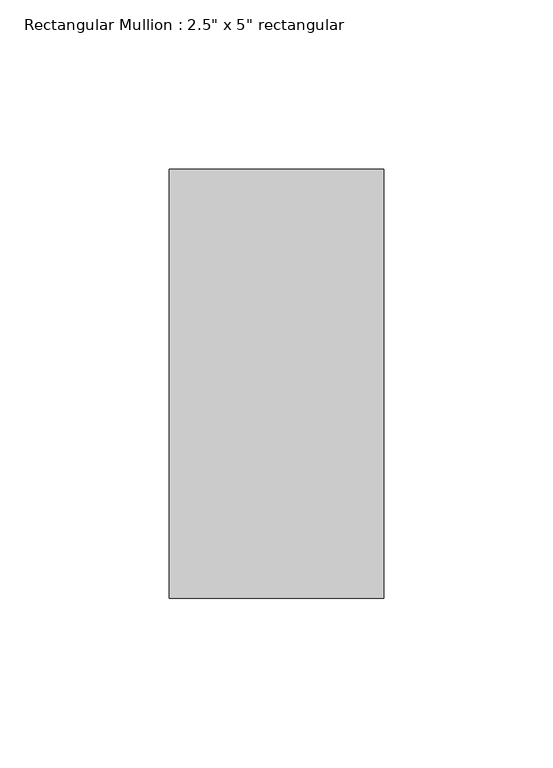
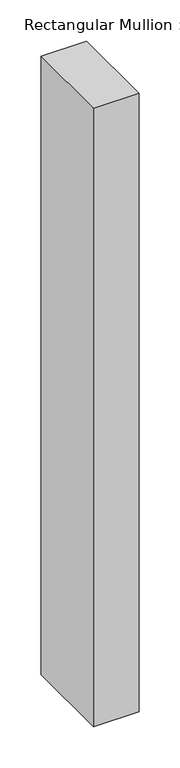
"""IFC4 building model written with IfcOpenShell, lengths in millimetres: member geometry."""

from ifc_helpers import new_model, si_unit, frame, origin, place, context, project, spatial, polyline, outline, extrude, source, transform, mapped, element, save


def member_410c6227(model_context):
    return source(origin(), model_context, "Body", "SweptSolid", [
        extrude(outline(polyline([(31.75, 63.5), (31.75, -63.5), (-31.75, -63.5), (-31.75, 63.5), (31.75, 63.5)])), frame((0.0, 0.0, -914.4), z_axis=(0.0, 0.0, 1.0), x_axis=(1.0, 0.0, 0.0)), (0.0, 0.0, 1.0), 914.4),
    ])


if __name__ == "__main__":
    model = new_model("IFC4")
    model_context = context("Model", 3, world=origin())
    ifc_project = project(units=[si_unit("LENGTHUNIT", "METRE", prefix="MILLI")], contexts=[model_context])
    site = spatial("IfcSite", under=ifc_project)
    building = spatial("IfcBuilding", under=site)
    placement = place(None, origin())
    member_shape = member_410c6227(model_context)
    element("IfcMember", 1, ObjectType="Rectangular Mullion : 2.5\" x 5\" rectangular", at=placement, inside=building, context=model_context, shape_type="MappedRepresentation", body=[
        mapped(member_shape, transform((0.0, 0.0, 0.0), x_axis=(1.0, 0.0, 0.0), y_axis=(0.0, 1.0, 0.0), z_axis=(0.0, 0.0, 1.0))),
    ])
    save(model, "model.ifc")

# Revit data of these elements
# Type "Rectangular Mullion : 2.5\" x 5\" rectangular"
#   built-in parameter 1007304 = 0.416667 (stored number, unit not read)
#   built-in parameter 1007301 = 0.104167 (stored number, unit not read)
#   built-in parameter 1007300 = 0.104167 (stored number, unit not read)
# Element 1 (IfcMember, "Rectangular Mullion : 2.5\" x 5\" rectangular")
#   Materials on its faces: "Iron, Ductile"
# Materials
#   "Iron, Ductile": class "Metal", colour RGB 0 0 0, transparency 0, Description = "Ductile cast iron", Cost = 0
